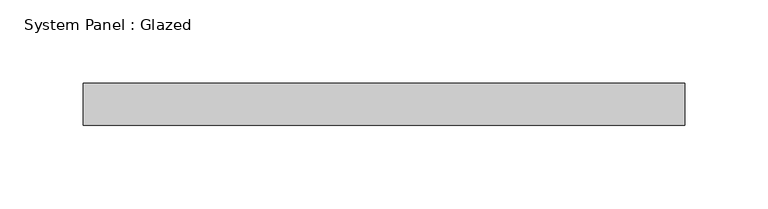
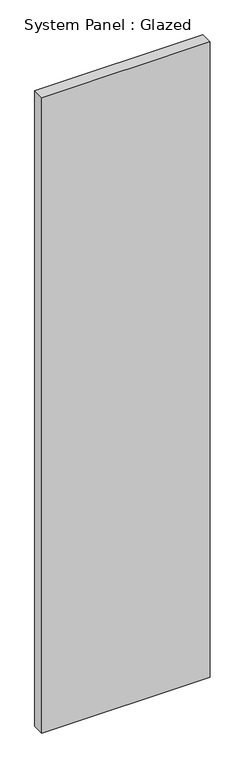
"""IFC4 building model written with IfcOpenShell, lengths in millimetres: plate geometry, System Panel : Glazed."""

from ifc_helpers import new_model, si_unit, origin, origin_with_axes, place, context, project, spatial, polyline, outline, extrude, source, transform, mapped, element, save


def system_panel_glazed_8adce2ad(model_context):
    return source(origin(), model_context, "Body", "SweptSolid", [
        extrude(outline(polyline([(180.975, 19.05), (-180.975, 19.05), (-180.975, 44.45), (180.975, 44.45), (180.975, 19.05)])), origin_with_axes(), (0.0, 0.0, 1.0), 1442.7635787),
    ])


if __name__ == "__main__":
    model = new_model("IFC4")
    model_context = context("Model", 3, world=origin())
    ifc_project = project(units=[si_unit("LENGTHUNIT", "METRE", prefix="MILLI")], contexts=[model_context])
    site = spatial("IfcSite", under=ifc_project)
    building = spatial("IfcBuilding", under=site)
    placement = place(None, origin())
    system_panel_glazed_shape = system_panel_glazed_8adce2ad(model_context)
    element("IfcPlate", 1, ObjectType="System Panel : Glazed", at=placement, inside=building, context=model_context, shape_type="MappedRepresentation", body=[
        mapped(system_panel_glazed_shape, transform((0.0, 0.0, 0.0), x_axis=(1.0, 0.0, 0.0), y_axis=(0.0, 1.0, 0.0), z_axis=(0.0, 0.0, 1.0))),
    ])
    save(model, "model.ifc")

# Revit data of these elements
# Type "System Panel : Glazed"
#   Construction Type Id = "GSP4R"
#   Analytic Construction = "1/8 in Pilkington single glazing"
#   Visual Light Transmittance = 0.9
#   Solar Heat Gain Coefficient = 0.86
#   Heat Transfer Coefficient (U) = 1.18115 BTU/(h·ft²·°F)
#   Define Thermal Properties by = 1
# Element 1 (IfcPlate, "System Panel : Glazed")
#   Materials on its faces: "Glass"
# Materials
#   "Glass": class "Glass", colour RGB 0 128 192, transparency 0.75, Description = "Soda Lime Glass", Cost = 0
